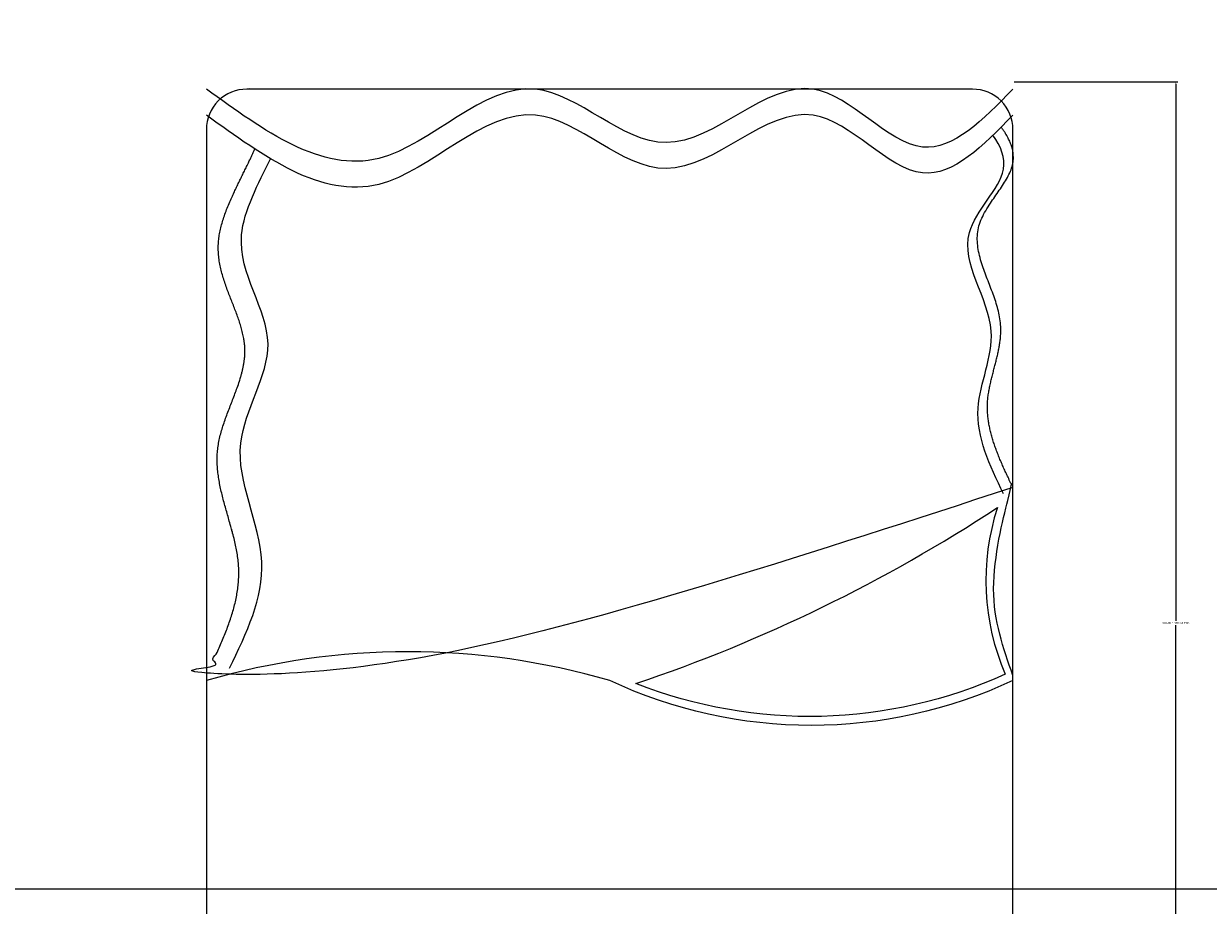
# Model space of a CAD drawing. Units: inches. Extents: x -61 to 1599, y -1316 to 257.
# Tile 9 of 204: x 99 to 200, y -1180 to -1105. Entities that reach past the tile are written whole.
import ezdxf

# ---------------------------------------------------------------- set-up
doc = ezdxf.new("R2010")
doc.units = ezdxf.units.IN
doc.header["$MEASUREMENT"] = 0
doc.layers.add('A-ANNO-DIMS', color=2, linetype='Continuous', lineweight=18)
doc.layers.add('FURNITURE', color=83, linetype='Continuous', lineweight=18)
doc.styles.get("Standard").update_dxf_attribs({"font": 'arial.ttf'})
doc.dimstyles.get("Standard").update_dxf_attribs({"dimtxt": 0.18, "dimasz": 0.18, "dimexe": 0.18, "dimexo": 0.0625, "dimgap": 0.09, "dimtad": 0, "dimtih": 1, "dimtoh": 1, "dimdec": 0, "dimzin": 0, "dimdsep": 46, "dimlunit": 3, "dimtxsty": 'Standard', "dimcen": 0.09, "dimadec": 0, "dimazin": 0, "dimtfac": 1, "dimtdec": 0, "dimtofl": 0, "dimtmove": 0, "dimatfit": 3, "dimfxl": 1, "dimtolj": 1, "dimtzin": 0, "dimarcsym": 0})

# ---------------------------------------------------------------- blocks, each defined once
blk = doc.blocks.new('BED-DOUBLE')
for points in [[(1.27, 88.54), (1.27, 3.45, 0.414214), (4.72, 0), (66.81, 0, 0.414214), (70.26, 3.45), (70.26, 88.54, 0.414214), (66.81, 91.99), (4.72, 91.99, 0.414214)], [(38.01, 41.13, 0.064396), (68.93, 56.18, 0.181766), (69.61, 41.92, -0.202767)]]:
    blk.add_lwpolyline(points, format="xyb", close=True)
blk.add_lwpolyline([(70.26, 41.39, -0.22309), (35.77, 41.39, 0.142156), (1.27, 41.39)], format="xyb")
for points, knots in [([(70.26, 91.99), (67.71, 89.38), (62.21, 83.76), (52.49, 96.72), (40.92, 82.74), (28.61, 96.74), (15.69, 81.53), (6.21, 88.41), (1.27, 91.99)], [0, 0, 0, 0, 9.176033, 19.753992, 33.150145, 45.209422, 59.881559, 75.764594, 75.764594, 75.764594, 75.764594]), ([(70.26, 89.76), (67.71, 87.16), (62.21, 81.54), (52.49, 94.5), (40.92, 80.52), (28.61, 94.52), (15.69, 79.31), (6.21, 86.19), (1.27, 89.76)], [0, 0, 0, 0, 9.176033, 19.753992, 33.150145, 45.209422, 59.881559, 75.764594, 75.764594, 75.764594, 75.764594]), ([(69.45, 57.36), (68.29, 59.79), (66.11, 64.34), (70.04, 71.91), (64.12, 79.11), (70.31, 84.4), (69.24, 87.09), (68.55, 88.05)], [0, 0, 0, 0, 6.649676, 12.451782, 19.973966, 25.324174, 28.349676, 28.349676, 28.349676, 28.349676]), ([(3.25, 42.44), (4.7, 45.45), (7.72, 51.72), (2.12, 61.25), (8.81, 70.52), (2.43, 77.93), (5.72, 83.91), (6.75, 86.04)], [0, 0, 0, 0, 8.27671, 17.241866, 24.903358, 33.244933, 38.427294, 38.427294, 38.427294, 38.427294])]:
    blk.add_open_spline(points, degree=3, knots=knots)
blk.add_open_spline([(5.01, 91.99), (4.99, 92.01), (4.96, 92.03), (4.94, 92.04)], degree=3)
for points, weights, knots in [([(70.26, 41.83), (68.02, 47.03), (68.02, 52.7), (70.26, 57.9), (69.1, 60.33), (66.92, 64.87), (70.85, 72.44), (64.93, 79.65), (71.19, 84.99), (70.01, 87.73), (69.25, 88.74)], [1, 0.945466318698, 0.945466318698, 1, 1, 1, 1, 1, 1, 1, 1], [0, 0, 0, 0, 0.814571, 0.814571, 0.814571, 7.464247, 13.266353, 20.788537, 26.138745, 29.321895, 29.321895, 29.321895, 29.321895]), ([(70.26, 57.9), (59.86, 50.94), (48.6, 45.5), (36.68, 41.68), (36.46, 41.77), (36.25, 41.87), (36.03, 41.97), (24.6, 45.28), (12.69, 45.26), (1.27, 41.89), (2.72, 44.9), (5.74, 51.17), (0.14, 60.7), (6.83, 69.97), (0.11, 77.79), (4.35, 84.38), (5.4, 86.88)], [1, 0.993520320424, 0.993520320424, 1, 0.99997444972, 0.99997444972, 1, 0.973174868659, 0.973174868659, 1, 1, 1, 1, 1, 1, 1, 1], [0, 0, 0, 0, 0.279074, 0.279074, 0.279074, 0.296584, 0.296584, 0.296584, 0.865868, 0.865868, 0.865868, 9.142578, 18.107734, 25.769226, 34.110801, 40.441511, 40.441511, 40.441511, 40.441511])]:
    blk.add_rational_spline(points, weights, degree=3, knots=knots)
blk = doc.blocks.new('*D634')
at = {"layer": 'A-ANNO-DIMS', "color": 0, "lineweight": -2, "transparency": 16777216}
for p, q in [((183.63, -1109.7), (197.64, -1109.7)), ((197.46, -1109.88), (197.46, -1155.83)), ((197.46, -1202.14), (197.46, -1156.19)), ((183.63, -1202.32), (197.64, -1202.32))]:
    blk.add_line(p, q, dxfattribs=at)
at = {"layer": 'A-ANNO-DIMS', "color": 0, "transparency": 16777216}
for points in [[(197.43, -1109.88), (197.49, -1109.88), (197.46, -1109.7)], [(197.43, -1202.14), (197.49, -1202.14), (197.46, -1202.32)]]:
    blk.add_solid(points, dxfattribs=at)
at = {"layer": 'DEFPOINTS', "color": 0, "transparency": 16777216}
for p in [(183.57, -1109.7), (197.46, -1109.7), (183.57, -1202.32)]:
    blk.add_point(p, dxfattribs=at)
at = {"layer": 'A-ANNO-DIMS', "color": 0, "transparency": 16777216, "insert": (197.46, -1156.01), "char_height": 0.18, "attachment_point": 5}
blk.add_mtext('\\A1;DOUBLE BED 93 TYP.', dxfattribs=at)
blk = doc.blocks.new('*D687')
at = {"layer": 'A-ANNO-DIMS', "color": 0, "lineweight": -2, "transparency": 16777216}
for p, q in [((289.42, 181.68), (-61.08, 181.68)), ((-60.9, 181.5), (-60.9, -528.95)), ((-60.9, -1239.76), (-60.9, -529.32)), ((319.64, -1239.94), (-61.08, -1239.94))]:
    blk.add_line(p, q, dxfattribs=at)
at = {"layer": 'A-ANNO-DIMS', "color": 0, "transparency": 16777216}
for points in [[(-60.93, 181.5), (-60.87, 181.5), (-60.9, 181.68)], [(-60.93, -1239.76), (-60.87, -1239.76), (-60.9, -1239.94)]]:
    blk.add_solid(points, dxfattribs=at)
at = {"layer": 'DEFPOINTS', "color": 0, "transparency": 16777216}
for p in [(289.48, 181.68), (-60.9, -1239.94), (319.7, -1239.94)]:
    blk.add_point(p, dxfattribs=at)
at = {"layer": 'A-ANNO-DIMS', "color": 0, "transparency": 16777216, "insert": (-60.9, -529.13), "char_height": 0.18, "attachment_point": 5}
blk.add_mtext('\\A1;1421.6', dxfattribs=at)
blk = doc.blocks.new('*D696')
at = {"layer": 'A-ANNO-DIMS', "color": 0, "lineweight": -2, "transparency": 16777216}
for p, q in [((690.64, -873.17), (-61.08, -873.17)), ((-60.9, -873.35), (-60.9, -1025.8)), ((-60.9, -1178.61), (-60.9, -1026.16)), ((690.64, -1178.79), (-61.08, -1178.79))]:
    blk.add_line(p, q, dxfattribs=at)
at = {"layer": 'A-ANNO-DIMS', "color": 0, "transparency": 16777216}
for points in [[(-60.93, -873.35), (-60.87, -873.35), (-60.9, -873.17)], [(-60.93, -1178.61), (-60.87, -1178.61), (-60.9, -1178.79)]]:
    blk.add_solid(points, dxfattribs=at)
at = {"layer": 'DEFPOINTS', "color": 0, "transparency": 16777216}
for p in [(-60.9, -873.17), (690.7, -873.17), (690.7, -1178.79)]:
    blk.add_point(p, dxfattribs=at)
at = {"layer": 'A-ANNO-DIMS', "color": 0, "transparency": 16777216, "insert": (-60.9, -1025.98), "char_height": 0.18, "attachment_point": 5}
blk.add_mtext('\\A1;305.6', dxfattribs=at)

msp = doc.modelspace()

# ---------------------------------------------------------------- block references
at = {"layer": 'FURNITURE'}
msp.add_blockref('BED-DOUBLE', (113.2612, -1202.3177), dxfattribs=at)

# ---------------------------------------------------------------- dimensions: what is measured, and where the dimension line sits
at = {"layer": 'A-ANNO-DIMS'}
for base, p1, p2, picture, middle in [((-60.8972, -1239.9446), (289.4807, 181.6771), (319.7028, -1239.9446), '*D687', (-60.8972, -529.1337)), ((-60.8972, -873.169), (690.7028, -1178.7933), (690.7028, -873.169), '*D696', (-60.8972, -1025.9812))]:
    dim = msp.add_linear_dim(base=base, p1=p1, p2=p2, angle=90, dimstyle='Standard', override={"dimdec": 1, "dimlfac": 1, "dimrnd": 0, "dimzin": 0, "dimdsep": 46, "dimlunit": 2}, dxfattribs=at)
    dim.commit()
    dim.dimension.update_dxf_attribs({"geometry": picture, "text_midpoint": middle})
dim = msp.add_linear_dim(base=(197.4625, -1109.6983), p1=(183.5695, -1202.3182), p2=(183.5695, -1109.6983), angle=90, text='DOUBLE BED <> TYP.', dimstyle='Standard', override={"dimdec": 0, "dimlfac": 1, "dimrnd": 0, "dimzin": 0, "dimdsep": 46, "dimlunit": 2}, dxfattribs=at)
dim.commit()
dim.dimension.update_dxf_attribs({"geometry": '*D634', "text_midpoint": (197.4625, -1156.0082)})

doc.saveas('drawing.dxf')
